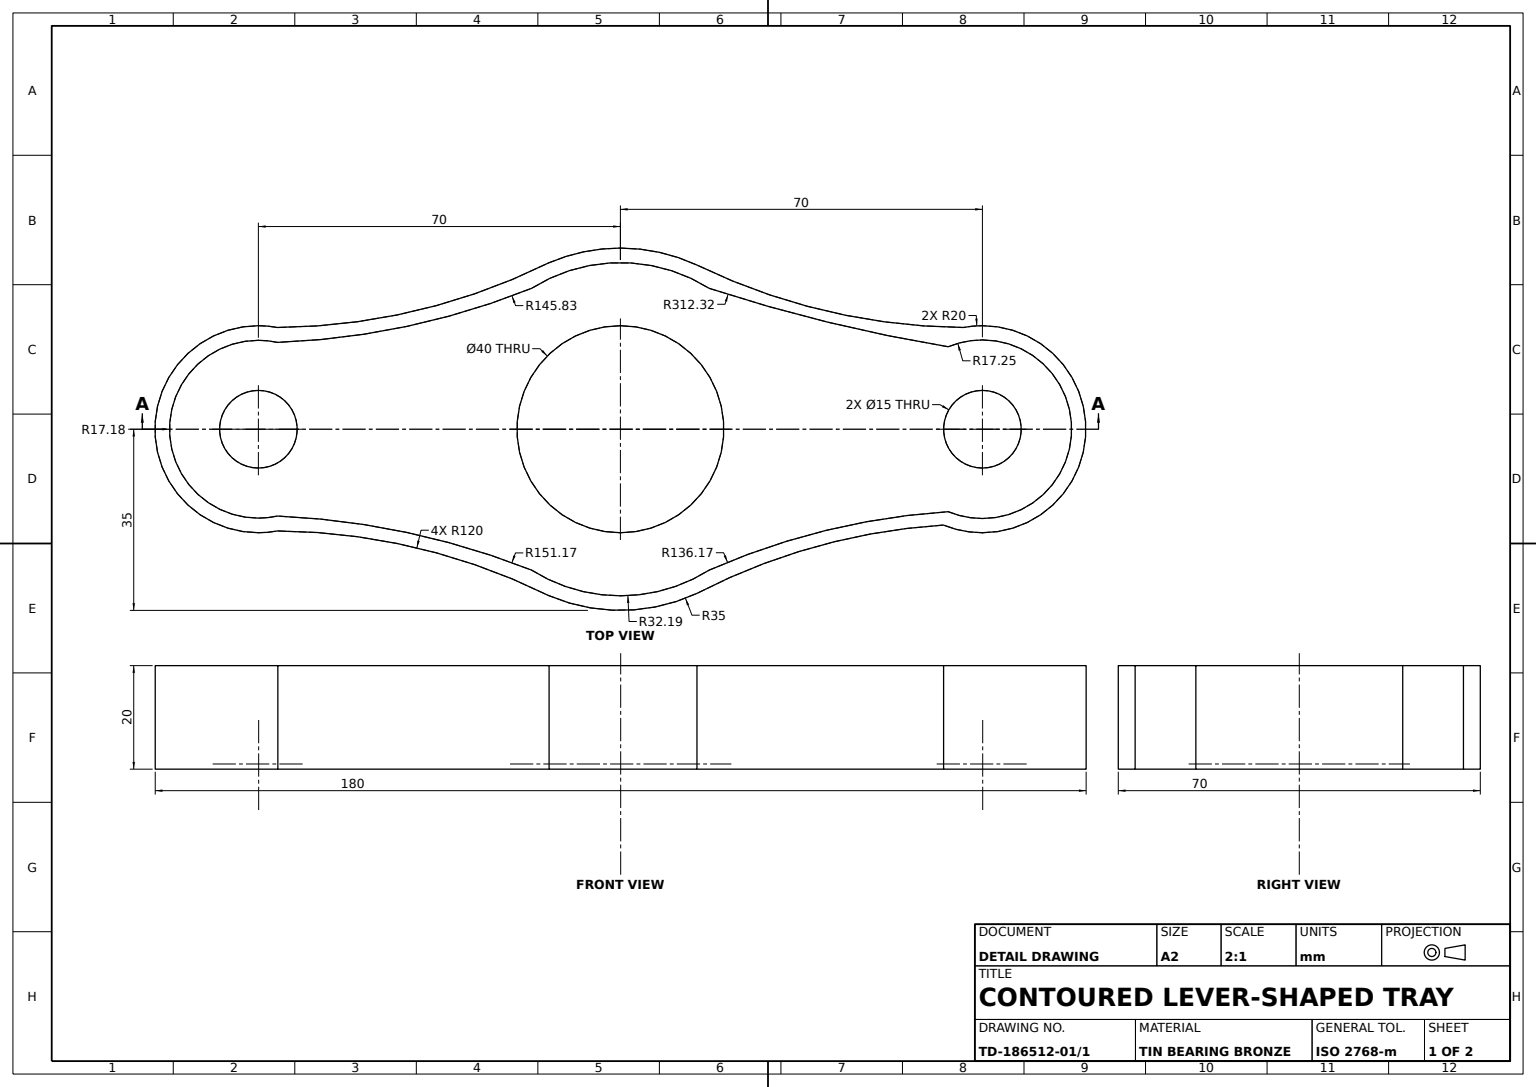
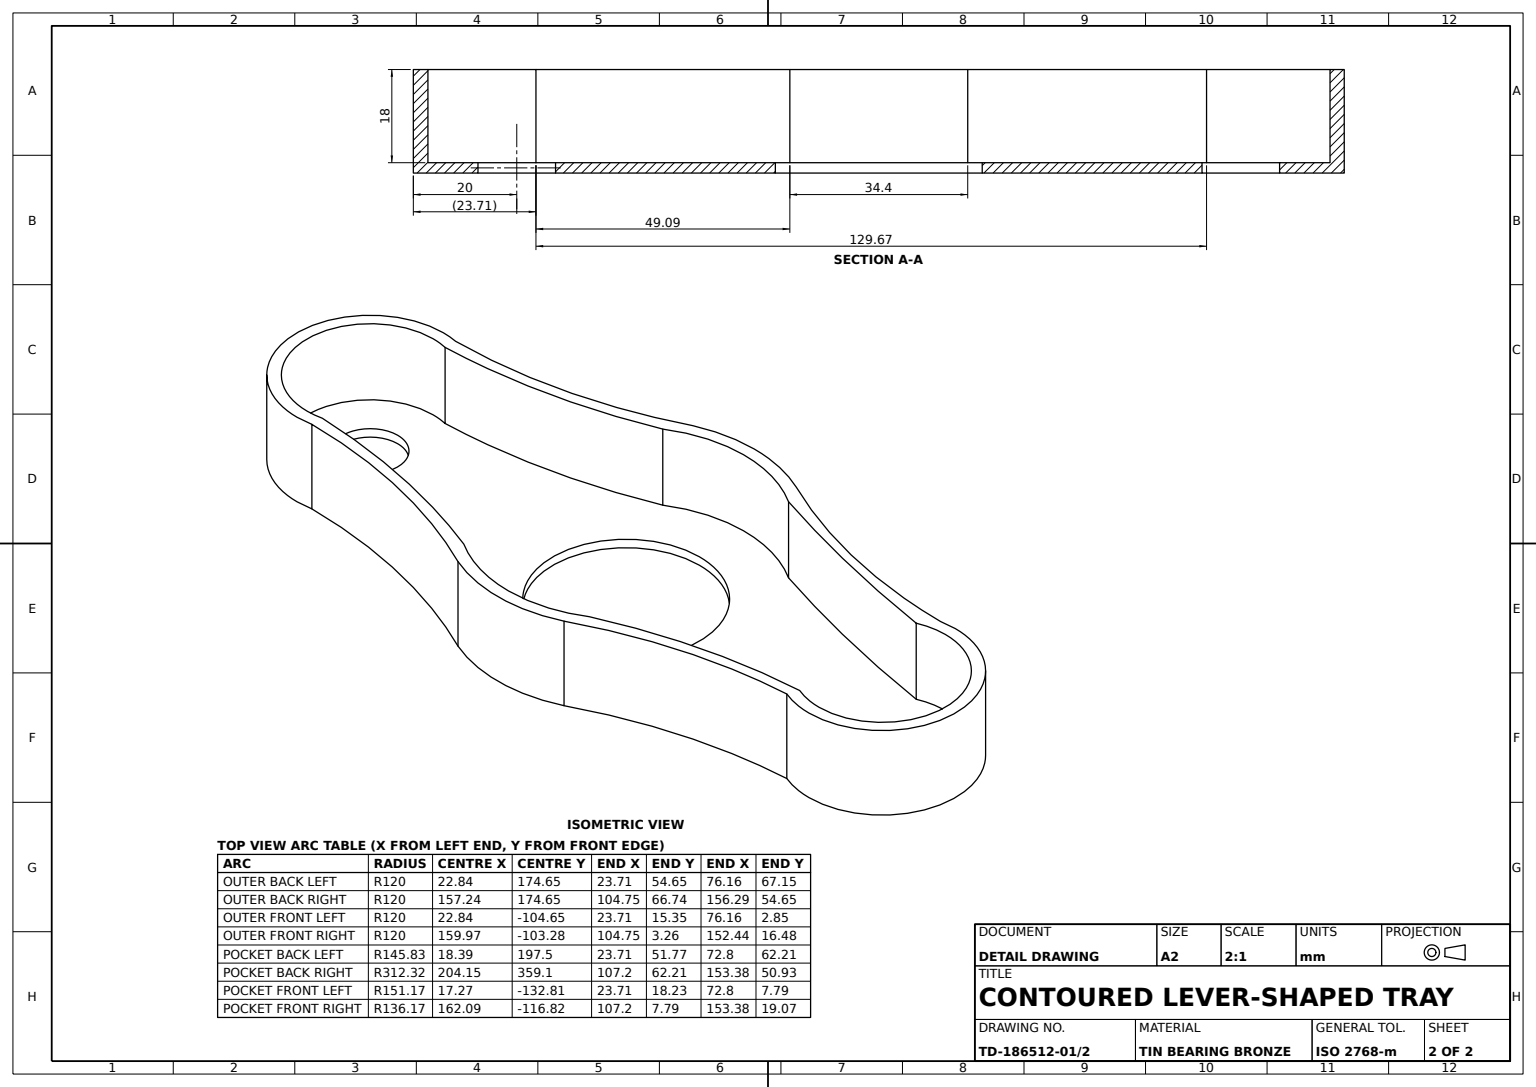
SolidWorks part; units mm, degrees
material "Tin Bearing Bronze"
ref_plane "Front Plane" through (0, 0, 0) normal (0, 0, 1) x (1, 0, 0)
ref_plane "Top Plane" through (0, 0, 0) normal (0, 1, 0) x (1, 0, 0)
ref_plane "Right Plane" through (0, 0, 0) normal (1, 0, 0) x (0, 0, -1)
sketch "Plate Outline and Holes Sketch" plane through (0, 0, 0) normal (0, 1, 0) x (1, 0, 0)
  line L0 (0, 0) -> (132.5812, 0) construction
  line L1 (66.2906, 0) -> (66.2906, -43.2345) construction
  line L2 (66.2906, -43.2345) -> (66.2906, 46.6752) construction
  circle A0 centre (66.2906, 0) radius 20
  circle A1 centre (136.2906, 0) radius 7.5
  circle A2 centre (-3.7094, 0) radius 7.5
  arc A3 (49.8206, -30.8827) -> (83.1295, -30.683) centre (66.2906, 0) ccw
  arc A4 (128.7307, -18.5162) -> (132.5812, 19.653) centre (136.2906, 0) ccw
  arc A5 (0, 19.653) -> (0, -19.653) centre (-3.7094, 0) ccw
  arc A6 (0, 19.653) -> (52.4479, 32.1462) centre (-0.8717, 139.6498) ccw
  arc A7 (0, -19.653) -> (52.4479, -32.1462) centre (-0.8717, -139.6498) cw
  arc A8 (81.0387, -31.741) -> (128.7307, -18.5162) centre (136.2612, -138.2797) cw
  arc A9 (81.0387, 31.741) -> (132.5812, 19.653) centre (133.5347, 139.6492) ccw
  arc A10 (81.9087, 31.3221) -> (49.8206, 30.8827) centre (66.2906, 0) ccw
  dimension "D1" = 40
  dimension "D2" = 15
  dimension "D3" = 15
  dimension "D5" = 120
  dimension "D6" = 40
  dimension "D7" = 40
  dimension "D8" = 120
  dimension "D9" = 120
  dimension "D10" = 120
  dimension "D15" = 35
  dimension "D4" = 140
  dimension "D11" = 132.5812
  dimension "D12" = 70
  dimension "D13" = 43.2345
  dimension "D14" = 89.9097
  dimension "D16" = 64.2925
  dimension "D17" = 18.5162
  dimension "D18" = 14.7481
extrude "Plate Body 20mm" add sketch "Plate Outline and Holes Sketch" along normal blind 20 contours A9 A10 A6 A5 A7 A3 A8 A4 A0 A1 A2
sketch "Pocket Outline Sketch" plane through (0, 20, 0) normal (0, 1, 0) x (1, 0, 0)
  line L0 (-3.7094, 0) -> (-3.7094, -28.5803) construction
  line L1 (136.2906, 0) -> (136.2906, -24.2884) construction
  arc A0 (0, 16.773) -> (0, -16.773) centre (-3.7094, 0) ccw
  arc A1 (129.6682, -15.9311) -> (129.6682, 15.9311) centre (136.2906, 0) ccw
  arc A2 (83.4883, 27.2063) -> (49.0929, 27.2063) centre (66.2906, 0) ccw
  arc A3 (0, 16.773) -> (49.0929, 27.2063) centre (-5.3154, 162.5021) ccw
  arc A4 (0, -16.773) -> (49.0929, -27.2063) centre (-6.4436, -167.8105) cw
  arc A5 (83.4883, -27.2063) -> (129.6682, -15.9311) centre (138.3794, -151.8179) cw
  arc A6 (83.4883, 27.2063) -> (129.6682, 15.9311) centre (180.4429, 324.0987) ccw
  arc A7 (49.0929, -27.2063) -> (83.4883, -27.2063) centre (66.2906, 0) ccw
  dimension "D1" = 17.1783
  dimension "D2" = 17.2527
  dimension "D3" = 32.186
  dimension "D4" = 145.826
  dimension "D5" = 151.1749
  dimension "D6" = 136.1657
  dimension "D7" = 312.3225
  dimension "D8" = 49.0929
  dimension "D9" = 129.6682
extrude "Pocket 18mm Deep" cut sketch "Pocket Outline Sketch" against normal blind 18
ref_plane "Plane3" through (81.0387, 0, 31.741) normal (0.9069, 0, -0.4214) x (-0.4214, 0, -0.9069)
